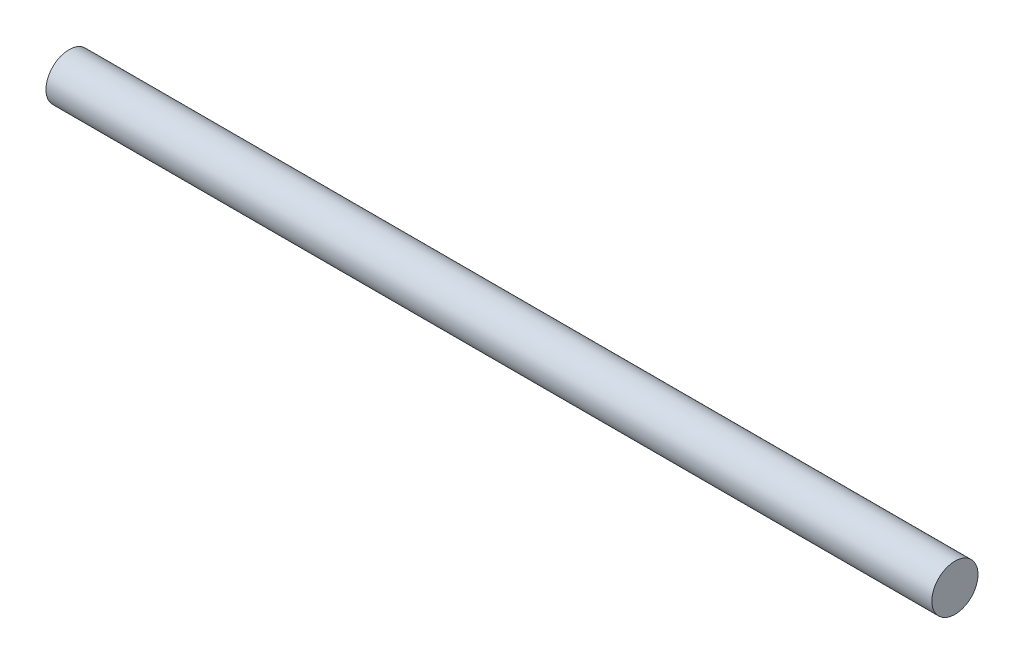
SolidWorks part; units mm, degrees
material "Plain Carbon Steel"
ref_plane "Front Plane" through (0, 0, 0) normal (0, 0, 1) x (1, 0, 0)
ref_plane "Top Plane" through (0, 0, 0) normal (0, 1, 0) x (1, 0, 0)
ref_plane "Right Plane" through (0, 0, 0) normal (1, 0, 0) x (0, 0, -1)
sketch "Rod Profile Ø5" plane through (0, 0, 0) normal (1, 0, 0) x (0, 0, -1)
  circle A0 centre (0, 0) radius 2.5
  dimension "D1" = 5
extrude "Rod Ø5x96" add sketch "Rod Profile Ø5" along normal blind 96
